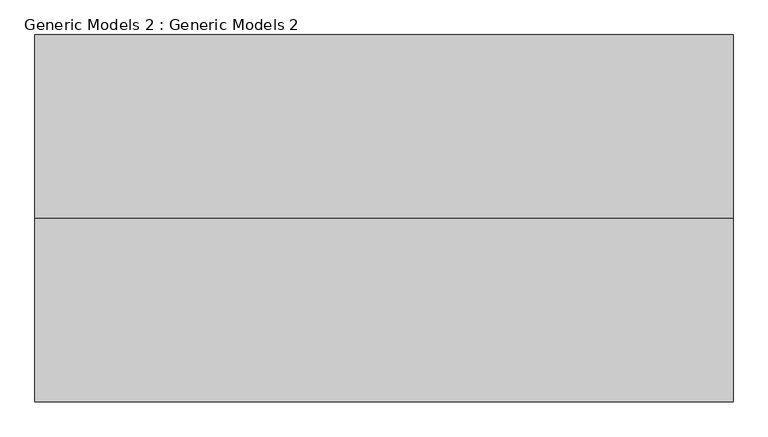
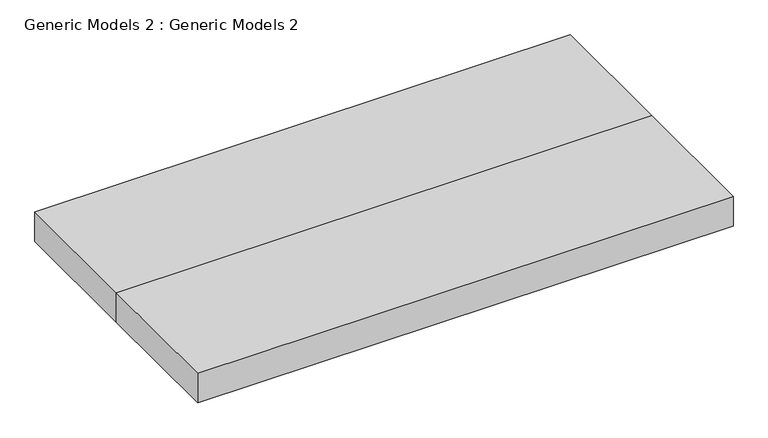
"""IFC4 building model written with IfcOpenShell, lengths in millimetres: proxy geometry, Generic Models 2 : Generic Models 2."""

from ifc_helpers import new_model, si_unit, origin, origin_with_axes, place, context, project, spatial, polyline, outline, extrude, source, transform, mapped, element, save


def generic_models_2_generic_models_2_0ca87cec(model_context):
    return source(origin(), model_context, "Body", "SweptSolid", [
        extrude(outline(polyline([(4419.6, 6819.2463046), (4419.6, 7140.1823212), (5638.8, 7140.1823212), (5638.8, 6819.2463046), (4419.6, 6819.2463046)])), origin_with_axes(), (0.0, 0.0, 1.0), 71.1016519),
        extrude(outline(polyline([(4419.6, 7140.1823212), (4419.6, 7461.1183378), (5638.8, 7461.1183378), (5638.8, 7140.1823212), (4419.6, 7140.1823212)])), origin_with_axes(), (0.0, 0.0, 1.0), 71.1016519),
    ])


if __name__ == "__main__":
    model = new_model("IFC4")
    model_context = context("Model", 3, world=origin())
    ifc_project = project(units=[si_unit("LENGTHUNIT", "METRE", prefix="MILLI")], contexts=[model_context])
    site = spatial("IfcSite", under=ifc_project)
    building = spatial("IfcBuilding", under=site)
    placement = place(None, origin())
    generic_models_2_generic_models_2_shape = generic_models_2_generic_models_2_0ca87cec(model_context)
    element("IfcBuildingElementProxy", 1, Name="Generic Models 2 : Generic Models 2", ObjectType="Generic Models 2 : Generic Models 2", at=placement, inside=building, context=model_context, shape_type="MappedRepresentation", body=[
        mapped(generic_models_2_generic_models_2_shape, transform((0.0, 0.0, 0.0), x_axis=(1.0, 0.0, 0.0), y_axis=(0.0, 1.0, 0.0), z_axis=(0.0, 0.0, 1.0))),
    ])
    save(model, "model.ifc")

# Revit data of these elements
# Element 1 (IfcBuildingElementProxy, "Generic Models 2 : Generic Models 2")
#   Materials on its faces: "Cherry", "Plywood, Sheathing", "Clad - White"
# Materials
#   "Cherry": class "Wood", colour RGB 226 177 128, transparency 0, Description = "Prunus Serotina", Cost = 0
#   "Plywood, Sheathing": class "Wood", colour RGB 212 179 113, transparency 0, Description = "Plywood, sheathing grade", Cost = 0
#   "Clad - White": class "Wood", colour RGB 242 242 238, transparency 0, Cost = 0
